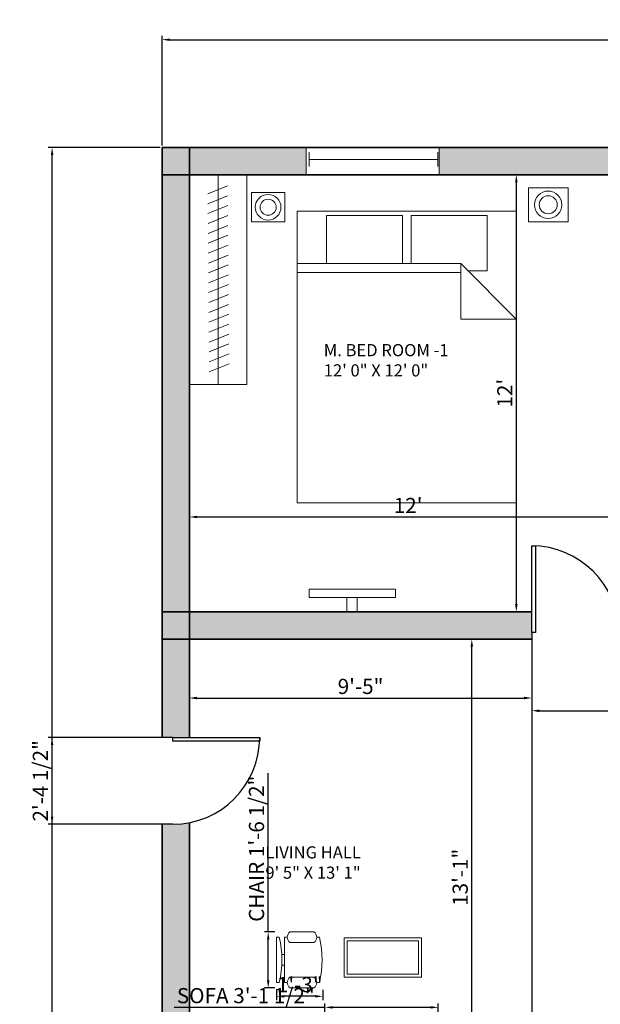
# Model space of a CAD drawing. Units: millimetres. Extents: x 2768 to 4359, y 795 to 1583.
# Tile 9 of 13: x 3572 to 3764, y 1258 to 1583. Entities that reach past the tile are written whole.
import ezdxf

# ---------------------------------------------------------------- set-up
doc = ezdxf.new("R2010")
doc.units = ezdxf.units.MM
for name, color, linetype, lineweight in [('A-ANNO-DIMS', 90, 'Continuous', 18), ('A-AREA-IDEN', 190, 'Continuous', 18), ('A-EQPM', 50, 'Continuous', 18), ('A-FLOR-CASE', 50, 'Continuous', 18), ('A-FLOR-CASE-PATT', 50, 'Continuous', 13), ('A-WALL-PATT', 140, 'Continuous', 9), ('doors', 10, 'Continuous', 25), ('furniture', 50, 'Continuous', 18), ('walls', 140, 'Continuous', 35), ('windows', 30, 'Continuous', 18)]:
    doc.layers.add(name, color=color, linetype=linetype, lineweight=lineweight)
doc.styles.get("Standard").update_dxf_attribs({"font": 'arial.ttf'})
doc.dimstyles.new('ISO-25', dxfattribs={"dimtxt": 5, "dimasz": 2.5, "dimexe": 1.25, "dimexo": 0.625, "dimtad": 1, "dimdec": 0, "dimlunit": 3, "dimtxsty": 'Standard', "dimcen": 2.5, "dimadec": 0, "dimazin": 0, "dimtfac": 1, "dimtdec": 0, "dimtmove": 0, "dimatfit": 3, "dimfxl": 1, "dimarcsym": 0})

# ---------------------------------------------------------------- blocks, each defined once
blk = doc.blocks.new('*U2')
for p, q in [((0, 0), (0, -6)), ((40, 0), (40, -6))]:
    blk.add_line(p, q)
blk.add_lwpolyline([(0, 0), (0, 40), (1.75, 40), (1.75, 0)], close=True)
blk.add_arc((0, 0), 40, 0, 90)
blk = doc.blocks.new('*U39')
for p, q in [((0, 4), (0, 0)), ((36, 4), (36, 0)), ((0, 2), (36, 2))]:
    blk.add_line(p, q)
blk = doc.blocks.new('Bed - Queen')
for p, q in [((0, -80.00003), (0, 0)), ((0, 0), (59.99999, 0)), ((59.99999, 0), (59.99999, -80.00003)), ((7.99999, -1.2), (28.79998, -1.2)), ((7.99999, -14.4), (7.99999, -1.2)), ((28.79998, -1.2), (28.79998, -14.4)), ((31.19999, -1.2), (51.99999, -1.2)), ((31.19999, -14.4), (31.19999, -1.2)), ((51.99999, -1.2), (51.99999, -16.4)), ((0, -14.4), (44.8, -14.4)), ((59.99999, -29.6), (44.8, -14.4)), ((44.8, -14.4), (44.8, -29.6)), ((44.8, -16.8), (0, -16.8)), ((51.99999, -16.4), (46.79936, -16.4)), ((44.8, -29.6), (59.99999, -29.6)), ((59.99999, -80.00003), (0, -80.00003))]:
    blk.add_line(p, q)
blk = doc.blocks.new('Chair - Desk')
for p, q in [((-8.5, 0), (-8.5, -1)), ((-8.5, 0), (8.5, 0)), ((8.5, 0), (8.5, -1)), ((-8.5, -3), (-8.5, -4)), ((-8.5, -3), (8.5, -3)), ((-2, -3), (-2, -1.9355)), ((2, -1.9576), (2, -3)), ((8.5, -3), (8.5, -4)), ((-10.5, -5), (-10.5, -14)), ((-6.5, -14), (-6.5, -5)), ((6.5, -5), (6.5, -14)), ((10.5, -14), (10.5, -5)), ((-8.5, -15), (-8.5, -16)), ((8.5, -15), (8.5, -16))]:
    blk.add_line(p, q)
for centre, radius, start, end in [((0, 34.625), 36.625, 256.5803, 283.4197), ((-8.5, -6.5), 2.5, 36.8699, 143.1301), ((8.5, -6.5), 2.5, 36.8699, 143.1301), ((-8.5, -12.5), 2.5, 216.8699, 323.1301), ((8.5, -12.5), 2.5, 216.8699, 323.1301), ((0, 19.625), 36.625, 256.5803, 283.4197)]:
    blk.add_arc(centre, radius, start, end)
blk = doc.blocks.new('*D40')
at = {"layer": 'A-ANNO-DIMS', "color": 0, "lineweight": -2, "transparency": 16777216}
for p, q in [((3628.37, 1418.42), (3628.37, 1417.79)), ((3630.87, 1419.04), (3769.87, 1419.04)), ((3772.37, 1419.67), (3772.37, 1420.29))]:
    blk.add_line(p, q, dxfattribs=at)
at = {"layer": 'A-ANNO-DIMS', "color": 0, "transparency": 16777216}
for points in [[(3630.87, 1419.46), (3630.87, 1418.62), (3628.37, 1419.04)], [(3769.87, 1419.46), (3769.87, 1418.62), (3772.37, 1419.04)]]:
    blk.add_solid(points, dxfattribs=at)
at = {"layer": 'Defpoints', "color": 0, "transparency": 16777216}
for p in [(3628.37, 1419.04), (3772.37, 1419.04), (3772.37, 1419.04)]:
    blk.add_point(p, dxfattribs=at)
at = {"layer": 'A-ANNO-DIMS', "color": 0, "transparency": 16777216, "insert": (3700.37, 1422.18), "char_height": 5, "attachment_point": 5}
blk.add_mtext("12'", dxfattribs=at)
blk = doc.blocks.new('*D41')
at = {"layer": 'A-ANNO-DIMS', "color": 0, "lineweight": -2, "transparency": 16777216}
for p, q in [((3732.45, 1531.81), (3737.26, 1531.81)), ((3736.01, 1529.31), (3736.01, 1390.31)), ((3736.63, 1387.81), (3737.26, 1387.81))]:
    blk.add_line(p, q, dxfattribs=at)
at = {"layer": 'A-ANNO-DIMS', "color": 0, "transparency": 16777216}
for points in [[(3735.59, 1529.31), (3736.43, 1529.31), (3736.01, 1531.81)], [(3735.59, 1390.31), (3736.43, 1390.31), (3736.01, 1387.81)]]:
    blk.add_solid(points, dxfattribs=at)
at = {"layer": 'Defpoints', "color": 0, "transparency": 16777216}
for p in [(3731.83, 1531.81), (3736.01, 1387.81), (3736.01, 1387.81)]:
    blk.add_point(p, dxfattribs=at)
at = {"layer": 'A-ANNO-DIMS', "color": 0, "transparency": 16777216, "insert": (3732.87, 1459.81), "char_height": 5, "attachment_point": 5, "rotation": 90}
blk.add_mtext("12'", dxfattribs=at)
blk = doc.blocks.new('*D49')
at = {"layer": 'A-ANNO-DIMS', "color": 0, "lineweight": -2, "transparency": 16777216}
for p, q in [((3628.37, 1378.18), (3628.37, 1358.13)), ((3741.08, 1376.03), (3741.08, 1358.13)), ((3630.87, 1359.38), (3738.58, 1359.38))]:
    blk.add_line(p, q, dxfattribs=at)
at = {"layer": 'A-ANNO-DIMS', "color": 0, "transparency": 16777216}
for points in [[(3630.87, 1359.8), (3630.87, 1358.96), (3628.37, 1359.38)], [(3738.58, 1359.8), (3738.58, 1358.96), (3741.08, 1359.38)]]:
    blk.add_solid(points, dxfattribs=at)
at = {"layer": 'Defpoints', "color": 0, "transparency": 16777216}
for p in [(3628.37, 1378.81), (3741.08, 1376.66), (3741.08, 1359.38)]:
    blk.add_point(p, dxfattribs=at)
at = {"layer": 'A-ANNO-DIMS', "color": 0, "transparency": 16777216, "insert": (3684.72, 1362.56), "char_height": 5, "attachment_point": 5}
blk.add_mtext('9\'-5"', dxfattribs=at)
blk = doc.blocks.new('*D50')
at = {"layer": 'A-ANNO-DIMS', "color": 0, "lineweight": -2, "transparency": 16777216}
for p, q in [((3727.24, 1378.81), (3720.1, 1378.81)), ((3721.35, 1224.31), (3721.35, 1376.31)), ((3727.24, 1221.81), (3720.1, 1221.81))]:
    blk.add_line(p, q, dxfattribs=at)
at = {"layer": 'A-ANNO-DIMS', "color": 0, "transparency": 16777216}
for points in [[(3720.94, 1376.31), (3721.77, 1376.31), (3721.35, 1378.81)], [(3720.94, 1224.31), (3721.77, 1224.31), (3721.35, 1221.81)]]:
    blk.add_solid(points, dxfattribs=at)
at = {"layer": 'Defpoints', "color": 0, "transparency": 16777216}
for p in [(3721.35, 1378.81), (3727.87, 1378.81), (3727.87, 1221.81)]:
    blk.add_point(p, dxfattribs=at)
at = {"layer": 'A-ANNO-DIMS', "color": 0, "transparency": 16777216, "insert": (3718.17, 1300.31), "char_height": 5, "attachment_point": 5, "rotation": 90}
blk.add_mtext('13\'-1"', dxfattribs=at)
blk = doc.blocks.new('*D64')
at = {"layer": 'A-ANNO-DIMS', "color": 0, "lineweight": -2, "transparency": 16777216}
for p, q in [((3910.37, 1364.28), (3910.37, 1353.94)), ((3741.08, 1357.5), (3741.08, 1353.94)), ((3743.58, 1355.19), (3907.87, 1355.19))]:
    blk.add_line(p, q, dxfattribs=at)
at = {"layer": 'A-ANNO-DIMS', "color": 0, "transparency": 16777216}
for points in [[(3743.58, 1355.61), (3743.58, 1354.77), (3741.08, 1355.19)], [(3907.87, 1355.61), (3907.87, 1354.77), (3910.37, 1355.19)]]:
    blk.add_solid(points, dxfattribs=at)
at = {"layer": 'Defpoints', "color": 0, "transparency": 16777216}
for p in [(3910.37, 1364.91), (3741.08, 1358.13), (3910.37, 1355.19)]:
    blk.add_point(p, dxfattribs=at)
at = {"layer": 'A-ANNO-DIMS', "color": 0, "transparency": 16777216, "insert": (3825.72, 1358.33), "char_height": 5, "attachment_point": 5}
blk.add_mtext('14\'-1"', dxfattribs=at)
blk = doc.blocks.new('*D89')
at = {"layer": 'A-ANNO-DIMS', "color": 0, "lineweight": -2, "transparency": 16777216}
for p, q in [((3654.32, 1282.32), (3654.32, 1334.63)), ((3656.47, 1282.32), (3653.07, 1282.32)), ((3654.32, 1266.37), (3654.32, 1279.82)), ((3656.47, 1263.87), (3653.07, 1263.87))]:
    blk.add_line(p, q, dxfattribs=at)
at = {"layer": 'A-ANNO-DIMS', "color": 0, "transparency": 16777216}
for points in [[(3653.91, 1279.82), (3654.74, 1279.82), (3654.32, 1282.32)], [(3653.91, 1266.37), (3654.74, 1266.37), (3654.32, 1263.87)]]:
    blk.add_solid(points, dxfattribs=at)
at = {"layer": 'Defpoints', "color": 0, "transparency": 16777216}
for p in [(3654.32, 1282.32), (3657.09, 1282.32), (3657.09, 1263.87)]:
    blk.add_point(p, dxfattribs=at)
at = {"layer": 'A-ANNO-DIMS', "color": 0, "transparency": 16777216, "insert": (3651.11, 1309.73), "char_height": 5, "attachment_point": 5, "rotation": 90}
blk.add_mtext('CHAIR 1\'-6 1/2"', dxfattribs=at)
blk = doc.blocks.new('*D90')
at = {"layer": 'A-ANNO-DIMS', "color": 0, "lineweight": -2, "transparency": 16777216}
for p, q in [((3657.09, 1263.24), (3657.09, 1259.85)), ((3672.33, 1263.24), (3672.33, 1259.85)), ((3669.83, 1261.1), (3659.59, 1261.1))]:
    blk.add_line(p, q, dxfattribs=at)
at = {"layer": 'A-ANNO-DIMS', "color": 0, "transparency": 16777216}
for points in [[(3659.59, 1261.51), (3659.59, 1260.68), (3657.09, 1261.1)], [(3669.83, 1261.51), (3669.83, 1260.68), (3672.33, 1261.1)]]:
    blk.add_solid(points, dxfattribs=at)
at = {"layer": 'Defpoints', "color": 0, "transparency": 16777216}
for p in [(3657.09, 1263.87), (3672.33, 1263.87), (3657.09, 1261.1)]:
    blk.add_point(p, dxfattribs=at)
at = {"layer": 'A-ANNO-DIMS', "color": 0, "transparency": 16777216, "insert": (3664.71, 1264.28), "char_height": 5, "attachment_point": 5}
blk.add_mtext('1\'-3"', dxfattribs=at)
blk = doc.blocks.new('*D105')
at = {"layer": 'A-ANNO-DIMS', "color": 0, "lineweight": -2, "transparency": 16777216}
for p, q in [((3673, 1257.45), (3623.37, 1257.45)), ((3673, 1252.49), (3673, 1258.7)), ((3707.79, 1257.45), (3675.5, 1257.45)), ((3710.29, 1252.49), (3710.29, 1258.7))]:
    blk.add_line(p, q, dxfattribs=at)
at = {"layer": 'A-ANNO-DIMS', "color": 0, "transparency": 16777216}
for points in [[(3675.5, 1257.87), (3675.5, 1257.04), (3673, 1257.45)], [(3707.79, 1257.87), (3707.79, 1257.04), (3710.29, 1257.45)]]:
    blk.add_solid(points, dxfattribs=at)
at = {"layer": 'Defpoints', "color": 0, "transparency": 16777216}
for p in [(3673, 1257.45), (3673, 1251.86), (3710.29, 1251.86)]:
    blk.add_point(p, dxfattribs=at)
at = {"layer": 'A-ANNO-DIMS', "color": 0, "transparency": 16777216, "insert": (3646.94, 1260.67), "char_height": 5, "attachment_point": 5}
blk.add_mtext('SOFA 3\'-1 1/2"', dxfattribs=at)
blk = doc.blocks.new('*D128')
at = {"layer": 'A-ANNO-DIMS', "color": 0, "lineweight": -2, "transparency": 16777216}
for p, q in [((3619.37, 1541.43), (3619.37, 1577.56)), ((4322.37, 1541.43), (4322.37, 1577.56)), ((3621.87, 1576.31), (4319.87, 1576.31))]:
    blk.add_line(p, q, dxfattribs=at)
at = {"layer": 'A-ANNO-DIMS', "color": 0, "transparency": 16777216}
for points in [[(3621.87, 1576.72), (3621.87, 1575.89), (3619.37, 1576.31)], [(4319.87, 1576.72), (4319.87, 1575.89), (4322.37, 1576.31)]]:
    blk.add_solid(points, dxfattribs=at)
at = {"layer": 'Defpoints', "color": 0, "transparency": 16777216}
for p in [(4322.37, 1576.31), (3619.37, 1540.81), (4322.37, 1540.81)]:
    blk.add_point(p, dxfattribs=at)
at = {"layer": 'A-ANNO-DIMS', "color": 0, "transparency": 16777216, "insert": (3970.87, 1579.49), "char_height": 5, "attachment_point": 5}
blk.add_mtext('58\'-7"', dxfattribs=at)
blk = doc.blocks.new('*D129')
at = {"layer": 'A-ANNO-DIMS', "color": 0, "lineweight": -2, "transparency": 16777216}
for p, q in [((3618.74, 1540.81), (3581.91, 1540.81)), ((3583.16, 837.66), (3583.16, 1538.31)), ((3618.74, 835.16), (3581.91, 835.16))]:
    blk.add_line(p, q, dxfattribs=at)
at = {"layer": 'A-ANNO-DIMS', "color": 0, "transparency": 16777216}
for points in [[(3582.75, 1538.31), (3583.58, 1538.31), (3583.16, 1540.81)], [(3582.75, 837.66), (3583.58, 837.66), (3583.16, 835.16)]]:
    blk.add_solid(points, dxfattribs=at)
at = {"layer": 'Defpoints', "color": 0, "transparency": 16777216}
for p in [(3583.16, 1540.81), (3619.37, 1540.81), (3619.37, 835.16)]:
    blk.add_point(p, dxfattribs=at)
at = {"layer": 'A-ANNO-DIMS', "color": 0, "transparency": 16777216, "insert": (3579.95, 1187.98), "char_height": 5, "attachment_point": 5, "rotation": 90}
blk.add_mtext('58\'-9 1/2"', dxfattribs=at)
blk = doc.blocks.new('*D132')
at = {"layer": 'A-ANNO-DIMS', "color": 0, "lineweight": -2, "transparency": 16777216}
for p, q in [((3618.74, 1346.39), (3581.91, 1346.39)), ((3583.16, 1320.31), (3583.16, 1343.89)), ((3618.74, 1317.81), (3581.91, 1317.81))]:
    blk.add_line(p, q, dxfattribs=at)
at = {"layer": 'A-ANNO-DIMS', "color": 0, "transparency": 16777216}
for points in [[(3582.75, 1343.89), (3583.58, 1343.89), (3583.16, 1346.39)], [(3582.75, 1320.31), (3583.58, 1320.31), (3583.16, 1317.81)]]:
    blk.add_solid(points, dxfattribs=at)
at = {"layer": 'Defpoints', "color": 0, "transparency": 16777216}
for p in [(3583.16, 1346.39), (3619.37, 1346.39), (3619.37, 1317.81)]:
    blk.add_point(p, dxfattribs=at)
at = {"layer": 'A-ANNO-DIMS', "color": 0, "transparency": 16777216, "insert": (3579.95, 1332.1), "char_height": 5, "attachment_point": 5, "rotation": 90}
blk.add_mtext('2\'-4 1/2"', dxfattribs=at)
blk = doc.blocks.new('*D135')
at = {"layer": 'A-ANNO-DIMS', "color": 0, "lineweight": -2, "transparency": 16777216}
for p, q in [((3741.08, 1378.18), (3741.08, 798.41)), ((3769.66, 1378.18), (3769.66, 798.41)), ((3743.58, 799.66), (3767.16, 799.66))]:
    blk.add_line(p, q, dxfattribs=at)
at = {"layer": 'A-ANNO-DIMS', "color": 0, "transparency": 16777216}
for points in [[(3743.58, 800.08), (3743.58, 799.24), (3741.08, 799.66)], [(3767.16, 800.08), (3767.16, 799.24), (3769.66, 799.66)]]:
    blk.add_solid(points, dxfattribs=at)
at = {"layer": 'Defpoints', "color": 0, "transparency": 16777216}
for p in [(3741.08, 1378.81), (3769.66, 1378.81), (3769.66, 799.66)]:
    blk.add_point(p, dxfattribs=at)
at = {"layer": 'A-ANNO-DIMS', "color": 0, "transparency": 16777216, "insert": (3755.37, 802.87), "char_height": 5, "attachment_point": 5}
blk.add_mtext('2\'-4 1/2"', dxfattribs=at)

msp = doc.modelspace()

# ---------------------------------------------------------------- hatches: boundary and pattern name
at = {"layer": 'A-FLOR-CASE-PATT'}
h = msp.add_hatch(dxfattribs=at)
h.set_pattern_fill('ANSI31', color=256, scale=0.954553, angle=-22.979, style=0)
h.paths.add_polyline_path([(3641.46, 1468.67), (3634.94, 1466.03), (3634.39, 1527.92), (3640.91, 1530.56)])
at = {"layer": 'A-WALL-PATT'}
h = msp.add_hatch(color=256, dxfattribs=at)
h.dxf.hatch_style = 1
h.paths.add_polyline_path([(3666.8, 1540.81), (3628.37, 1540.81), (3628.37, 1531.81), (3666.8, 1531.81)])
h.paths.add_polyline_path([(3628.37, 1540.81), (3619.37, 1540.81), (3619.37, 1531.81), (3628.37, 1531.81)])
h.paths.add_polyline_path([(3628.37, 1531.81), (3619.37, 1531.81), (3619.37, 1387.81), (3628.37, 1387.81)])
h.paths.add_polyline_path([(3772.37, 1540.81), (3710.62, 1540.81), (3710.62, 1531.81), (3772.37, 1531.81)])
h.paths.add_polyline_path([(3796.31, 1540.81), (3781.37, 1540.81), (3781.37, 1531.81), (3796.31, 1531.81)])
h.paths.add_polyline_path([(3781.37, 1540.81), (3772.37, 1540.81), (3772.37, 1531.81), (3781.37, 1531.81)])
h.paths.add_polyline_path([(3781.37, 1531.81), (3772.37, 1531.81), (3772.37, 1493.05), (3773.51, 1493.08), (3781.37, 1493.27)])
h.paths.add_polyline_path([(3841.37, 1540.81), (3822.12, 1540.81), (3822.12, 1531.81), (3841.37, 1531.81)])
h.paths.add_polyline_path([(3867.29, 1540.81), (3850.37, 1540.81), (3850.37, 1531.81), (3867.29, 1531.81)])
h.paths.add_polyline_path([(3850.37, 1540.81), (3841.37, 1540.81), (3841.37, 1531.81), (3850.37, 1531.81)])
h.paths.add_polyline_path([(3850.37, 1531.81), (3841.37, 1531.81), (3841.37, 1435.81), (3850.37, 1435.81)])
h.paths.add_polyline_path([(3919.37, 1531.81), (3910.37, 1531.81), (3910.37, 1495.39, -0.097322), (3918.93, 1497.3), (3919.37, 1497.31)])
h.paths.add_polyline_path([(3919.37, 1540.81), (3910.37, 1540.81), (3910.37, 1531.81), (3919.37, 1531.81)])
h.paths.add_polyline_path([(3910.37, 1540.81), (3893.19, 1540.81), (3893.19, 1531.81), (3910.37, 1531.81)])
h.paths.add_polyline_path([(3971.85, 1540.81), (3919.37, 1540.81), (3919.37, 1531.81), (3971.85, 1531.81)])
h.paths.add_polyline_path([(4063.37, 1540.81), (4017.44, 1540.81), (4017.44, 1531.81), (4063.37, 1531.81)])
h.paths.add_polyline_path([(4072.37, 1531.81), (4063.37, 1531.81), (4063.37, 1387.81), (4072.37, 1387.81)])
h.paths.add_polyline_path([(4072.37, 1378.81), (4063.37, 1378.81), (4063.37, 1240.81), (4072.37, 1240.81)])
h.paths.add_polyline_path([(4072.37, 1387.81), (4063.37, 1387.81), (4063.37, 1378.81), (4072.37, 1378.81)])
h.paths.add_polyline_path([(3919.37, 1387.81), (3910.37, 1387.81), (3910.37, 1378.81), (3919.37, 1378.81)])
h.paths.add_polyline_path([(3919.37, 1392.95, -0.05459), (3913.18, 1392.28), (3910.37, 1392.28), (3910.37, 1387.81), (3919.37, 1387.81)])
h.paths.add_polyline_path([(3919.37, 1474.55), (3910.37, 1474.32), (3910.37, 1435.81), (3919.37, 1435.81)])
h.paths.add_polyline_path([(3919.37, 1435.81), (3910.37, 1435.81), (3910.37, 1426.81), (3919.37, 1426.81)])
h.paths.add_polyline_path([(3910.37, 1435.81), (3850.37, 1435.81), (3850.37, 1426.81), (3910.37, 1426.81)])
h.paths.add_polyline_path([(3919.37, 1426.81), (3910.37, 1426.81), (3910.37, 1420.86), (3913.18, 1420.86), (3919.37, 1420.86)])
h.paths.add_polyline_path([(3850.37, 1435.81), (3841.37, 1435.81), (3841.37, 1426.81), (3850.37, 1426.81)])
h.paths.add_polyline_path([(3841.37, 1435.81), (3781.37, 1435.81), (3781.37, 1426.81), (3841.37, 1426.81)])
h.paths.add_polyline_path([(3781.37, 1435.81), (3772.37, 1435.81), (3772.37, 1426.81), (3781.37, 1426.81)])
h.paths.add_polyline_path([(3781.37, 1426.81), (3772.37, 1426.81), (3772.37, 1420.59, -0.050492), (3778.09, 1421.17), (3781.37, 1421.17)])
h.paths.add_polyline_path([(3781.37, 1471.72, -0.082137), (3774.07, 1470.33), (3772.37, 1470.29), (3772.37, 1435.81), (3781.37, 1435.81)])
h.paths.add_polyline_path([(3628.37, 1387.81), (3619.37, 1387.81), (3619.37, 1378.81), (3628.37, 1378.81)])
h.paths.add_polyline_path([(3628.37, 1378.81), (3619.37, 1378.81), (3619.37, 1346.39), (3622.95, 1346.39), (3628.37, 1346.39)])
h.paths.add_polyline_path([(3781.37, 1387.81), (3772.37, 1387.81), (3772.37, 1378.81), (3781.37, 1378.81)])
h.paths.add_polyline_path([(3781.37, 1392.59), (3778.09, 1392.59), (3772.37, 1392.59), (3772.37, 1387.81), (3781.37, 1387.81)])
h.paths.add_polyline_path([(3628.37, 1318.32, -0.047705), (3622.95, 1317.81), (3619.37, 1317.81), (3619.37, 1221.81), (3628.37, 1221.81)])
h.paths.add_polyline_path([(3628.37, 1221.81), (3619.37, 1221.81), (3619.37, 1212.81), (3628.37, 1212.81)])
h.paths.add_polyline_path([(3827.37, 1221.81), (3628.37, 1221.81), (3628.37, 1212.81), (3827.37, 1212.81)])
h.paths.add_polyline_path([(3628.37, 1212.81), (3619.37, 1212.81), (3619.37, 1116.81), (3628.37, 1116.81)])
h.paths.add_polyline_path([(3836.37, 1221.81), (3827.37, 1221.81), (3827.37, 1212.81), (3836.37, 1212.81)])
h.paths.add_polyline_path([(3628.37, 1107.81), (3619.37, 1107.81), (3619.37, 1047.81), (3628.37, 1047.81)])
h.paths.add_polyline_path([(3628.37, 1116.81), (3619.37, 1116.81), (3619.37, 1107.81), (3628.37, 1107.81)])
h.paths.add_polyline_path([(3836.37, 1155.81), (3827.37, 1155.81), (3827.37, 1116.81), (3836.37, 1116.81)])
h.paths.add_polyline_path([(3836.37, 1116.81), (3827.37, 1116.81), (3827.37, 1107.81), (3836.37, 1107.81)])
h.paths.add_polyline_path([(3836.37, 1107.81), (3827.37, 1107.81), (3827.37, 1047.81), (3836.37, 1047.81)])
h.paths.add_polyline_path([(3827.37, 1047.37), (3827.37, 1047.81), (3739.96, 1047.81), (3739.96, 1038.81), (3827.37, 1038.81)])
h.paths.add_polyline_path([(3836.37, 1047.37), (3836.37, 1047.81), (3827.37, 1047.81), (3827.37, 1047.37), (3827.37, 1038.81), (3836.37, 1038.81)])
h.paths.add_polyline_path([(3695.08, 1047.81), (3628.37, 1047.81), (3628.37, 1038.81), (3695.08, 1038.81)])
h.paths.add_polyline_path([(3628.37, 1047.81), (3619.37, 1047.81), (3619.37, 1038.81), (3628.37, 1038.81)])
h.paths.add_polyline_path([(3850.59, 1047.81), (3836.37, 1047.81), (3836.37, 1047.37), (3836.37, 1038.81), (3850.59, 1038.81)])
h.paths.add_polyline_path([(3896.37, 1047.37), (3896.37, 1047.81), (3876.26, 1047.81), (3876.26, 1038.81), (3896.37, 1038.81)])
h.paths.add_polyline_path([(3905.37, 1109.65), (3903.46, 1109.6), (3896.37, 1109.43), (3896.37, 1047.81), (3905.37, 1047.81)])
h.paths.add_polyline_path([(3905.37, 1047.81), (3896.37, 1047.81), (3896.37, 1047.37), (3896.37, 1038.81), (3905.37, 1038.81)])
h.paths.add_polyline_path([(4063.37, 1047.81), (3905.37, 1047.81), (3905.37, 1038.81), (4063.37, 1038.81)])
h.paths.add_polyline_path([(4072.37, 1137.28), (4063.37, 1137.28), (4063.37, 1047.81), (4072.37, 1047.81)])
h.paths.add_polyline_path([(4072.37, 1231.81), (4063.37, 1231.81), (4063.37, 1182.55), (4072.37, 1182.55)])
h.paths.add_polyline_path([(4072.37, 1240.81), (4063.37, 1240.81), (4063.37, 1231.81), (4072.37, 1231.81)])
h.paths.add_polyline_path([(4072.37, 1047.81), (4063.37, 1047.81), (4063.37, 1038.81), (4072.37, 1038.81)])
h.paths.add_polyline_path([(3905.37, 1231.81), (3896.37, 1231.81), (3896.37, 1164.81), (3905.37, 1164.81)])
h.paths.add_polyline_path([(3905.37, 1240.81), (3896.37, 1240.81), (3896.37, 1231.81), (3905.37, 1231.81)])
h.paths.add_polyline_path([(3910.61, 1237.57), (3910.61, 1240.81), (3905.37, 1240.81), (3905.37, 1231.81), (3911.2, 1231.81, -0.050754)])
h.paths.add_polyline_path([(3988.37, 1240.81), (3939.19, 1240.81), (3939.19, 1237.57), (3939.19, 1231.81), (3988.37, 1231.81)])
h.paths.add_polyline_path([(3997.37, 1240.81), (3988.37, 1240.81), (3988.37, 1231.81), (3997.37, 1231.81)])
h.paths.add_polyline_path([(4063.37, 1240.81), (3997.37, 1240.81), (3997.37, 1231.81), (4063.37, 1231.81)])
h.paths.add_polyline_path([(3997.37, 1334.21), (3988.37, 1334.21), (3988.37, 1288.44), (3997.37, 1288.44)])
h.paths.add_polyline_path([(3896.37, 1164.81), (3836.37, 1164.81), (3836.37, 1155.81), (3896.37, 1155.81)])
h.paths.add_polyline_path([(3836.37, 1164.81), (3827.37, 1164.81), (3827.37, 1155.81), (3836.37, 1155.81)])
h.paths.add_polyline_path([(3905.37, 1164.81), (3896.37, 1164.81), (3896.37, 1155.81), (3905.37, 1155.81)])
h.paths.add_polyline_path([(3905.37, 1155.81), (3896.37, 1155.81), (3896.37, 1131.22, -0.073168), (3902.89, 1132.35), (3905.37, 1132.41)])
edge = h.paths.add_edge_path()
edge.add_line((3951.89, 1380.74), (3951.89, 1378.81))
edge.add_line((3951.89, 1378.81), (4063.37, 1378.81))
edge.add_line((4063.37, 1378.81), (4063.37, 1387.81))
edge.add_line((4063.37, 1387.81), (3951, 1387.81))
edge.add_arc((3923.31, 1380.74), 28.58, 0, 14.3236, ccw=False)
h.paths.add_polyline_path([(3923.31, 1378.81), (3923.31, 1387.81), (3919.37, 1387.81), (3919.37, 1378.81)])
edge = h.paths.add_edge_path()
edge.add_arc((3775.74, 1114.53), 22.75, 187.4686, 197.1843)
edge.add_line((3754, 1107.81), (3628.37, 1107.81))
edge.add_line((3628.37, 1107.81), (3628.37, 1116.81))
edge.add_line((3628.37, 1116.81), (3752.42, 1116.81))
edge.add_arc((3775.17, 1117.41), 22.75, 181.5276, 194.8757)
h.paths.add_polyline_path([(3775.68, 1116.81), (3775.91, 1107.81), (3827.37, 1107.81), (3827.37, 1116.81)])
h = msp.add_hatch(color=256, dxfattribs=at)
h.dxf.hatch_style = 1
h.paths.add_polyline_path([(3628.37, 1387.81), (3628.37, 1378.81), (3741.08, 1378.81), (3741.08, 1380.94), (3741.08, 1387.81)])
h.paths.add_polyline_path([(3769.66, 1380.94), (3769.66, 1378.81), (3772.37, 1378.81), (3772.37, 1387.81), (3768.82, 1387.81, -0.060722)])

# ---------------------------------------------------------------- linework, layer by layer
at = {"layer": 'A-EQPM'}
for points in [[(3667.76, 1392.51), (3696.25, 1392.51), (3696.25, 1395.28), (3667.76, 1395.28)], [(3680.22, 1387.81), (3683.6, 1387.81), (3683.6, 1392.53), (3680.22, 1392.53)]]:
    msp.add_lwpolyline(points, close=True, dxfattribs=at)
at = {"layer": 'A-FLOR-CASE'}
msp.add_line((3637.85, 1462.68), (3637.85, 1531.81), dxfattribs=at)
msp.add_lwpolyline([(3628.37, 1531.81), (3647.33, 1531.81), (3647.33, 1462.68), (3628.37, 1462.68)], close=True, dxfattribs=at)
at = {"layer": 'furniture'}
for points in [[(3648.81, 1525.94), (3659.77, 1525.94), (3659.77, 1516.26), (3648.81, 1516.26)], [(3740.01, 1527.51), (3753.03, 1527.51), (3753.03, 1516.32), (3740.01, 1516.32)], [(3679.3, 1280.41), (3704.77, 1280.41), (3704.77, 1267.38), (3679.3, 1267.38)], [(3680.3, 1279.41), (3703.77, 1279.41), (3703.77, 1268.38), (3680.3, 1268.38)]]:
    msp.add_lwpolyline(points, close=True, dxfattribs=at)
for centre, radius in [((3654.29, 1521.1), 4.22), ((3746.52, 1521.92), 4.51), ((3746.52, 1521.92), 2.98), ((3654.29, 1521.1), 2.65)]:
    msp.add_circle(centre, radius, dxfattribs=at)
at = {"layer": 'walls'}
for p, q in [((3619.37, 1540.81), (3619.37, 1346.39)), ((3619.37, 1540.81), (4322.37, 1540.81)), ((3628.37, 1540.81), (3628.37, 1346.39)), ((3619.37, 1531.81), (4322.37, 1531.81)), ((3619.37, 1387.81), (3741.08, 1387.81)), ((3619.37, 1387.81), (3741.08, 1387.81)), ((3619.37, 1378.81), (3741.08, 1378.81)), ((3619.37, 1378.81), (3741.08, 1378.81)), ((3619.37, 1317.81), (3619.37, 835.16)), ((3628.37, 1318.32), (3628.37, 835.16))]:
    msp.add_line(p, q, dxfattribs=at)
at = {"layer": 'windows'}
for p, q in [((3666.8, 1540.81), (3666.8, 1531.81)), ((3710.62, 1540.81), (3710.62, 1531.81))]:
    msp.add_line(p, q, dxfattribs=at)

# ---------------------------------------------------------------- block references
at = {"layer": 'doors', "xscale": 0.7144929449846577, "yscale": 0.7144929449846577, "zscale": 0.7144929449846577}
msp.add_blockref('*U2', (3741.08, 1380.94), dxfattribs=at)
at = {"layer": 'doors', "xscale": 0.7144929449846577, "yscale": 0.7144929449846577, "zscale": 0.7144929449846577, "rotation": 270}
msp.add_blockref('*U2', (3622.95, 1346.39), dxfattribs=at)
at = {"layer": 'furniture', "xscale": 1.201893325172568, "yscale": 1.201893325172568, "zscale": 1.201893325172568}
msp.add_blockref('Bed - Queen', (3663.9, 1519.83), dxfattribs=at)
at = {"layer": 'furniture', "xscale": 0.8789788586979289, "yscale": 0.8789788586979289, "zscale": 0.8789788586979289, "rotation": 90}
msp.add_blockref('Chair - Desk', (3657.09, 1273.1), dxfattribs=at)
at = {"layer": 'windows', "xscale": 1.175999919670228, "yscale": 1.175999919670228, "zscale": 1.175999919670228}
msp.add_blockref('*U39', (3667.79, 1534.5), dxfattribs=at)

# ---------------------------------------------------------------- texts
at = {"layer": 'A-AREA-IDEN', "char_height": 4, "attachment_point": 1}
for s, width, insert in [('M. BED ROOM -1 \\P12\' 0" X 12\' 0"', 53.3594, (3672.62, 1476.01)), ('LIVING HALL \\P9\' 5" X 13\' 1"', 38.7972, (3653.39, 1310.52))]:
    msp.add_mtext_dynamic_manual_height_columns(s, width=width, gutter_width=12.5, heights=[0], dxfattribs=dict(at, insert=insert))

# ---------------------------------------------------------------- dimensions: what is measured, and where the dimension line sits
at = {"layer": 'A-ANNO-DIMS'}
for base, p1, p2, override, picture, middle in [((4322.37, 1576.31), (3619.37, 1540.81), (4322.37, 1540.81), {"dimdec": 1, "dimlfac": 1, "dimrnd": 0, "dimzin": 1, "dimdsep": 46, "dimlunit": 4, "dimfrac": 2}, '*D128', (3970.87, 1579.49)), ((3772.37, 1419.04), (3628.37, 1419.04), (3772.37, 1419.04), {"dimclrd": 0, "dimclre": 0, "dimclrt": 0}, '*D40', (3700.37, 1422.18)), ((3741.08, 1359.38), (3628.37, 1378.81), (3741.08, 1376.66), {"dimclrd": 0, "dimclre": 0, "dimclrt": 0}, '*D49', (3684.72, 1362.56)), ((3769.66, 799.66), (3741.08, 1378.81), (3769.66, 1378.81), {"dimdec": 1, "dimlfac": 1, "dimrnd": 0, "dimzin": 1, "dimdsep": 46, "dimlunit": 4, "dimfrac": 2}, '*D135', (3755.37, 802.87)), ((3910.37, 1355.19), (3741.08, 1358.13), (3910.37, 1364.91), {"dimclrd": 0, "dimclre": 0, "dimclrt": 0}, '*D64', (3825.72, 1358.33))]:
    dim = msp.add_linear_dim(base=base, p1=p1, p2=p2, dimstyle='ISO-25', override=override, dxfattribs=at)
    dim.commit()
    dim.dimension.update_dxf_attribs({"geometry": picture, "text_midpoint": middle})
for base, p1, p2, angle, override, picture, middle in [((3583.1625, 1540.8077), (3619.366, 835.1598), (3619.366, 1540.8077), 90, {"dimdec": 1, "dimlfac": 1, "dimrnd": 0, "dimzin": 1, "dimdsep": 46, "dimlunit": 4, "dimfrac": 2}, '*D129', (3579.9523, 1187.9838)), ((3736.01, 1387.81), (3731.83, 1531.81), (3736.01, 1387.81), 90, {"dimclrd": 0, "dimclre": 0, "dimclrt": 0}, '*D41', (3732.87, 1459.81)), ((3721.35, 1378.81), (3727.87, 1221.81), (3727.87, 1378.81), 90, {"dimclrd": 0, "dimclre": 0, "dimclrt": 0}, '*D50', (3718.17, 1300.31)), ((3583.16, 1346.39), (3619.37, 1317.81), (3619.37, 1346.39), 90, {"dimdec": 1, "dimlfac": 1, "dimrnd": 0, "dimzin": 1, "dimdsep": 46, "dimlunit": 4, "dimfrac": 2}, '*D132', (3579.95, 1332.1)), ((3657.09, 1261.1), (3672.33, 1263.87), (3657.09, 1263.87), 180, {"dimdec": 1, "dimlfac": 1, "dimrnd": 0, "dimzin": 1, "dimdsep": 46, "dimlunit": 4, "dimfrac": 2}, '*D90', (3664.71, 1264.28))]:
    dim = msp.add_linear_dim(base=base, p1=p1, p2=p2, angle=angle, dimstyle='ISO-25', override=override, dxfattribs=at)
    dim.commit()
    dim.dimension.update_dxf_attribs({"geometry": picture, "text_midpoint": middle})
for base, p1, p2, angle, text, picture, middle in [((3654.3243, 1282.3245), (3657.0931, 1263.8659), (3657.0931, 1282.3245), 90, 'CHAIR <>', '*D89', (3651.1141, 1309.7281)), ((3673, 1257.45), (3710.29, 1251.86), (3673, 1251.86), 180, 'SOFA <>', '*D105', (3646.94, 1260.67))]:
    dim = msp.add_linear_dim(base=base, p1=p1, p2=p2, angle=angle, text=text, dimstyle='ISO-25', override={"dimdec": 1, "dimlfac": 1, "dimrnd": 0, "dimzin": 1, "dimdsep": 46, "dimlunit": 4, "dimfrac": 2}, dxfattribs=at)
    dim.commit()
    dim.dimension.update_dxf_attribs({"geometry": picture, "text_midpoint": middle})

doc.saveas('drawing.dxf')
